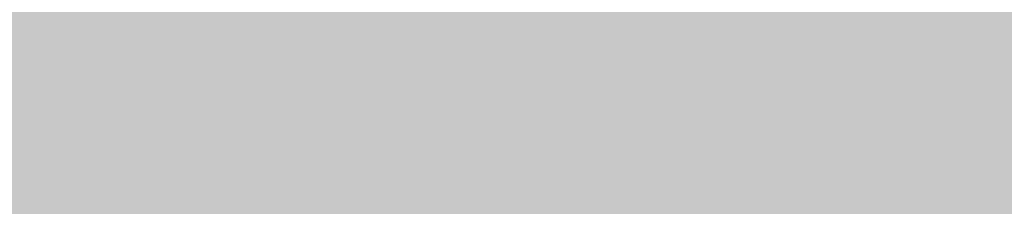
# Model space of a CAD drawing. Units: millimetres. Extents: x 0 to 2267, y 0 to 1823.
# Tile 49 of 256: x 1595.098 to 1596.855, y 1226.386 to 1226.718. Entities that reach past the tile are written whole.
import ezdxf

# ---------------------------------------------------------------- set-up
doc = ezdxf.new("R2010")
doc.units = ezdxf.units.MM
doc.header["$MEASUREMENT"] = 0
doc.layers.add('M-HATC', color=252, linetype='Continuous', lineweight=18)

msp = doc.modelspace()

# ---------------------------------------------------------------- hatches: boundary and pattern name
at = {"layer": 'M-HATC'}
h = msp.add_hatch(color=256, dxfattribs=at)
h.dxf.hatch_style = 1
h.paths.add_polyline_path([(2055.771, 1603.062), (1381.0868, 1603.062), (1381.0868, 1598.062), (2055.771, 1598.062)])
h.paths.add_polyline_path([(2055.771, 1598.062), (1381.0868, 1598.062), (1381.0868, 1593.062), (2055.771, 1593.062)])
h.paths.add_polyline_path([(2051.3074, 1536.7609), (1385.5504, 1536.7609), (1385.5504, 1526.7609), (1387.5504, 1526.7609), (1388.5366, 1525.0528), (1385.3319, 1521.2335), (1385.3319, 1521.2226), (2050.2542, 1522.7491), (2048.3212, 1525.0528), (2049.3074, 1526.7609), (2051.3074, 1526.7609)])
edge = h.paths.add_edge_path()
edge.add_arc((1847.5345, 1379.1492), 135, 222.603061, 222.890851, ccw=False)
edge.add_line((1748.1663, 1287.7656), (1683.0921, 1287.7656))
edge.add_arc((1583.7239, 1379.1492), 135, 317.109149, 317.396939, ccw=False)
edge.add_arc((1678.9686, 1290.6707), 5, 222.8909, 317.1091, ccw=False)
edge.add_arc((1774.2133, 1379.1492), 135, 222.603061, 222.890851, ccw=False)
edge.add_line((1674.8451, 1287.7656), (1609.7709, 1287.7656))
edge.add_arc((1510.4027, 1379.1492), 135, 317.109149, 317.396939, ccw=False)
edge.add_arc((1605.6474, 1290.6707), 5, 222.8909, 317.1091, ccw=False)
edge.add_arc((1700.8921, 1379.1492), 135, 222.603061, 222.890851, ccw=False)
edge.add_line((1601.5239, 1287.7656), (1536.4497, 1287.7656))
edge.add_arc((1437.0815, 1379.1492), 135, 317.109149, 317.396939, ccw=False)
edge.add_arc((1532.3262, 1290.6707), 5, 222.8909, 317.1091, ccw=False)
edge.add_arc((1627.5709, 1379.1492), 135, 222.603061, 222.890851, ccw=False)
edge.add_line((1528.2027, 1287.7656), (1505.9289, 1287.7656))
edge.add_spline(control_points=[(1505.9289, 1287.7656), (1504.2622, 1287.7656), (1504.2622, 1282.7656), (1505.9289, 1282.7656)], knot_values=[0, 0, 0, 0, 5, 5, 5, 5], degree=3, periodic=0)
edge.add_line((1505.9289, 1282.7656), (1930.9289, 1282.7656))
edge.add_spline(control_points=[(1930.9289, 1282.7656), (1932.5956, 1282.7656), (1932.5956, 1287.7656), (1930.9289, 1287.7656)], knot_values=[0, 0, 0, 0, 5, 5, 5, 5], degree=3, periodic=0)
edge.add_line((1930.9289, 1287.7656), (1903.0557, 1287.7656))
edge.add_arc((1803.6875, 1379.1492), 135, 317.109149, 317.396939, ccw=False)
edge.add_arc((1898.9322, 1290.6707), 5, 222.8909, 317.1091, ccw=False)
edge.add_arc((1994.1769, 1379.1492), 135, 222.603061, 222.890851, ccw=False)
edge.add_line((1894.8087, 1287.7656), (1829.7345, 1287.7656))
edge.add_arc((1730.3663, 1379.1492), 135, 317.109149, 317.396939, ccw=False)
edge.add_arc((1825.611, 1290.6707), 5, 222.8909, 317.1091, ccw=False)
edge.add_arc((1920.8557, 1379.1492), 135, 222.603061, 222.890851, ccw=False)
edge.add_line((1821.4875, 1287.7656), (1756.4133, 1287.7656))
edge.add_arc((1657.0451, 1379.1492), 135, 317.109149, 317.396939, ccw=False)
edge.add_arc((1752.2898, 1290.6707), 5, 222.8909, 317.1091, ccw=False)
edge = h.paths.add_edge_path()
edge.add_spline(control_points=[(1843.4289, 1227.2475), (1845.0956, 1227.2475), (1845.0956, 1232.2475), (1843.4289, 1232.2475)], knot_values=[0, 0, 0, 0, 5, 5, 5, 5], degree=3, periodic=0)
edge.add_line((1843.4289, 1232.2475), (1593.4289, 1232.2475))
edge.add_spline(control_points=[(1593.4289, 1232.2475), (1591.7622, 1232.2475), (1591.7622, 1227.2475), (1593.4289, 1227.2475)], knot_values=[0, 0, 0, 0, 5, 5, 5, 5], degree=3, periodic=0)
edge.add_line((1593.4289, 1227.2475), (1843.4289, 1227.2475))
h.paths.add_polyline_path([(1905.9289, 1127.4171), (1530.9289, 1127.4171, 0.414214), (1520.9289, 1117.4171), (1530.9289, 1117.4171), (1915.9289, 1117.4171, 0.414214)])
edge = h.paths.add_edge_path()
edge.add_arc((1397.0858, 1498.4078), 12.7299, 90.78215, 190.87871, ccw=False)
edge.add_line((1396.912, 1511.1365), (1428.0097, 1511.3488))
edge.add_line((1428.0097, 1511.3488), (1433.0097, 1511.3488))
edge.add_line((1433.0097, 1511.3488), (1434.439, 1511.3488))
edge.add_arc((1419.474, 1498.0804), 20, 41.561, 74.08211)
edge.add_line((1424.9592, 1517.3135), (1399.9351, 1517.2561))
edge.add_spline(control_points=[(1399.9307, 1517.2561), (1399.884, 1517.2131), (1399.8328, 1517.1689), (1399.7774, 1517.1236)], knot_values=[11.567499, 11.567499, 11.567499, 11.567499, 11.814249, 11.814249, 11.814249, 11.814249], degree=3, periodic=0)
edge.add_spline(control_points=[(1399.6328, 1517.0099), (1399.5831, 1516.9721), (1399.5307, 1516.9338), (1399.4759, 1516.8947)], knot_values=[11.167718, 11.167718, 11.167718, 11.167718, 11.365188, 11.365188, 11.365188, 11.365188], degree=3, periodic=0)
edge.add_spline(control_points=[(1399.3398, 1516.8001), (1399.1514, 1516.6719), (1398.9384, 1516.5377), (1398.704, 1516.3994)], knot_values=[10.376405, 10.376405, 10.376405, 10.376405, 11.00994, 11.00994, 11.00994, 11.00994], degree=3, periodic=0)
edge.add_spline(control_points=[(1398.6572, 1516.3719), (1398.5789, 1516.326), (1398.4983, 1516.2797), (1398.4155, 1516.2331)], knot_values=[10.125175, 10.125175, 10.125175, 10.125175, 10.334406, 10.334406, 10.334406, 10.334406], degree=3, periodic=0)
edge.add_spline(control_points=[(1398.2642, 1516.1487), (1398.196, 1516.1111), (1398.1263, 1516.0732), (1398.0555, 1516.0351)], knot_values=[9.832246, 9.832246, 9.832246, 9.832246, 9.999658, 9.999658, 9.999658, 9.999658], degree=3, periodic=0)
edge.add_spline(control_points=[(1397.9987, 1516.0048), (1397.7312, 1515.8621), (1397.446, 1515.7171), (1397.1466, 1515.5714)], knot_values=[9.161808, 9.161808, 9.161808, 9.161808, 9.787769, 9.787769, 9.787769, 9.787769], degree=3, periodic=0)
edge.add_spline(control_points=[(1397.1466, 1515.5714), (1396.8418, 1515.423), (1396.5222, 1515.274), (1396.1914, 1515.1262)], knot_values=[8.524455, 8.524455, 8.524455, 8.524455, 9.161808, 9.161808, 9.161808, 9.161808], degree=3, periodic=0)
edge.add_spline(control_points=[(1396.0777, 1515.0756), (1395.9854, 1515.0348), (1395.8922, 1514.994), (1395.7983, 1514.9534)], knot_values=[8.275193, 8.275193, 8.275193, 8.275193, 8.451726, 8.451726, 8.451726, 8.451726], degree=3, periodic=0)
edge.add_spline(control_points=[(1395.6018, 1514.8691), (1395.4997, 1514.8257), (1395.3968, 1514.7824), (1395.2932, 1514.7394)], knot_values=[7.962917, 7.962917, 7.962917, 7.962917, 8.152764, 8.152764, 8.152764, 8.152764], degree=3, periodic=0)
edge.add_spline(control_points=[(1395.2116, 1514.7057), (1394.8278, 1514.5475), (1394.4345, 1514.3929), (1394.0364, 1514.2442)], knot_values=[7.21254, 7.21254, 7.21254, 7.21254, 7.913148, 7.913148, 7.913148, 7.913148], degree=3, periodic=0)
edge.add_spline(control_points=[(1394.0364, 1514.2442), (1393.7076, 1514.1214), (1393.3754, 1514.0027), (1393.0427, 1513.8895)], knot_values=[6.633733, 6.633733, 6.633733, 6.633733, 7.21254, 7.21254, 7.21254, 7.21254], degree=3, periodic=0)
edge.add_spline(control_points=[(1392.8214, 1513.815), (1392.7198, 1513.7812), (1392.6181, 1513.7479), (1392.5166, 1513.7152)], knot_values=[6.328796, 6.328796, 6.328796, 6.328796, 6.505493, 6.505493, 6.505493, 6.505493], degree=3, periodic=0)
edge.add_spline(control_points=[(1392.5166, 1513.7152), (1392.3187, 1513.6515), (1392.1212, 1513.59), (1391.9244, 1513.531)], knot_values=[5.984605, 5.984605, 5.984605, 5.984605, 6.328796, 6.328796, 6.328796, 6.328796], degree=3, periodic=0)
edge.add_spline(control_points=[(1391.7915, 1513.4915), (1391.3122, 1513.3501), (1390.8384, 1513.2239), (1390.3784, 1513.1171)], knot_values=[5.066697, 5.066697, 5.066697, 5.066697, 5.907055, 5.907055, 5.907055, 5.907055], degree=3, periodic=0)
edge.add_spline(control_points=[(1390.3784, 1513.1171), (1390.1797, 1513.071), (1389.9836, 1513.0284), (1389.7907, 1512.9899)], knot_values=[4.70367, 4.70367, 4.70367, 4.70367, 5.066695, 5.066695, 5.066695, 5.066695], degree=3, periodic=0)
edge.add_spline(control_points=[(1389.422, 1512.9204), (1389.2459, 1512.8892), (1389.0729, 1512.8617), (1388.9036, 1512.8381)], knot_values=[4.130571, 4.130571, 4.130571, 4.130571, 4.469816, 4.469816, 4.469816, 4.469816], degree=3, periodic=0)
edge.add_spline(control_points=[(1388.9036, 1512.8381), (1388.591, 1512.7946), (1388.2911, 1512.7644), (1388.0071, 1512.7494)], knot_values=[3.504031, 3.504031, 3.504031, 3.504031, 4.130571, 4.130571, 4.130571, 4.130571], degree=3, periodic=0)
edge.add_spline(control_points=[(1387.9356, 1512.7459), (1387.8538, 1512.7423), (1387.7733, 1512.74), (1387.6944, 1512.739)], knot_values=[3.268866, 3.268866, 3.268866, 3.268866, 3.451164, 3.451164, 3.451164, 3.451164], degree=3, periodic=0)
edge.add_spline(control_points=[(1387.3351, 1512.7443), (1387.2076, 1512.7499), (1387.0847, 1512.7597), (1386.967, 1512.7739)], knot_values=[2.670686, 2.670686, 2.670686, 2.670686, 2.984, 2.984, 2.984, 2.984], degree=3, periodic=0)
edge.add_spline(control_points=[(1386.8327, 1512.7922), (1386.8209, 1512.7941), (1386.8092, 1512.7959), (1386.7975, 1512.7979)], knot_values=[2.516981, 2.516981, 2.516981, 2.516981, 2.549528, 2.549528, 2.549528, 2.549528], degree=3, periodic=0)
edge.add_spline(control_points=[(1386.4526, 1512.8735), (1386.4257, 1512.881), (1386.3993, 1512.889), (1386.3733, 1512.8972)], knot_values=[2.095869, 2.095869, 2.095869, 2.095869, 2.17941, 2.17941, 2.17941, 2.17941], degree=3, periodic=0)
edge.add_spline(control_points=[(1386.0691, 1513.0189), (1386.0634, 1513.0217), (1386.0577, 1513.0246), (1386.052, 1513.0275)], knot_values=[1.72453, 1.72453, 1.72453, 1.72453, 1.745933, 1.745933, 1.745933, 1.745933], degree=3, periodic=0)
edge.add_arc((1399.474, 1498.0804), 20, 131.82432, 180)
edge.add_arc((1630.3336, 1505.5484), 250.9708, 181.705176, 236.427975)
edge.add_arc((1605.3399, 1483.3044), 218.7822, 238.660829, 243.34961)
edge.add_arc((1647.0911, 1510.3592), 262.8986, 183.129836, 237.853442, ccw=False)
h.paths.add_polyline_path([(1406.5369, 1391.9644, 0.149382), (1491.5506, 1296.4418, -0.129517)], flags=17)
edge = h.paths.add_edge_path()
edge.add_arc((2037.3838, 1498.0804), 20, 0, 48.26587)
edge.add_spline(control_points=[(2050.6973, 1513.0052), (2050.6512, 1512.9847), (2050.6034, 1512.9655), (2050.5539, 1512.9477)], knot_values=[1.835652, 1.835652, 1.835652, 1.835652, 2.000781, 2.000781, 2.000781, 2.000781], degree=3, periodic=0)
edge.add_spline(control_points=[(2050.4616, 1512.9166), (2050.479, 1512.9221), (2050.4963, 1512.9277), (2050.5133, 1512.9335)], knot_values=[2.045477, 2.045477, 2.045477, 2.045477, 2.101389, 2.101389, 2.101389, 2.101389], degree=3, periodic=0)
edge.add_spline(control_points=[(2050.129, 1512.8342), (2050.1984, 1512.8473), (2050.2657, 1512.8623), (2050.3308, 1512.8792)], knot_values=[2.237629, 2.237629, 2.237629, 2.237629, 2.435841, 2.435841, 2.435841, 2.435841], degree=3, periodic=0)
edge.add_spline(control_points=[(2050.0946, 1512.8278), (2050.1061, 1512.8299), (2050.1176, 1512.832), (2050.129, 1512.8342)], knot_values=[2.435841, 2.435841, 2.435841, 2.435841, 2.468321, 2.468321, 2.468321, 2.468321], degree=3, periodic=0)
edge.add_spline(control_points=[(2049.7843, 1512.7851), (2049.8552, 1512.7922), (2049.9243, 1512.8008), (2049.9917, 1512.8109)], knot_values=[2.563852, 2.563852, 2.563852, 2.563852, 2.748541, 2.748541, 2.748541, 2.748541], degree=3, periodic=0)
edge.add_spline(control_points=[(2049.4052, 1512.7617), (2049.5364, 1512.7653), (2049.6629, 1512.773), (2049.7843, 1512.7851)], knot_values=[2.748541, 2.748541, 2.748541, 2.748541, 3.064882, 3.064882, 3.064882, 3.064882], degree=3, periodic=0)
edge.add_spline(control_points=[(2049.1698, 1512.7597), (2049.2336, 1512.7591), (2049.2965, 1512.7594), (2049.3584, 1512.7606)], knot_values=[3.102309, 3.102309, 3.102309, 3.102309, 3.2503, 3.2503, 3.2503, 3.2503], degree=3, periodic=0)
edge.add_spline(control_points=[(2048.8573, 1512.7691), (2048.9638, 1512.7638), (2049.068, 1512.7606), (2049.1698, 1512.7597)], knot_values=[3.2503, 3.2503, 3.2503, 3.2503, 3.486069, 3.486069, 3.486069, 3.486069], degree=3, periodic=0)
edge.add_spline(control_points=[(2048.6924, 1512.7789), (2048.3729, 1512.8009), (2048.0345, 1512.8411), (2047.6817, 1512.897)], knot_values=[3.606429, 3.606429, 3.606429, 3.606429, 4.2989, 4.2989, 4.2989, 4.2989], degree=3, periodic=0)
edge.add_spline(control_points=[(2047.6817, 1512.897), (2047.5458, 1512.9185), (2047.4077, 1512.9424), (2047.2678, 1512.9685)], knot_values=[4.2989, 4.2989, 4.2989, 4.2989, 4.565769, 4.565769, 4.565769, 4.565769], degree=3, periodic=0)
edge.add_spline(control_points=[(2047.2678, 1512.9685), (2047.1449, 1512.9914), (2047.0207, 1513.016), (2046.8951, 1513.0422)], knot_values=[4.565769, 4.565769, 4.565769, 4.565769, 4.799971, 4.799971, 4.799971, 4.799971], degree=3, periodic=0)
edge.add_spline(control_points=[(2046.8951, 1513.0422), (2046.5286, 1513.1188), (2046.1513, 1513.209), (2045.7676, 1513.3107)], knot_values=[4.799971, 4.799971, 4.799971, 4.799971, 5.483718, 5.483718, 5.483718, 5.483718], degree=3, periodic=0)
edge.add_spline(control_points=[(2045.7676, 1513.3107), (2045.3724, 1513.4154), (2044.9704, 1513.5322), (2044.5662, 1513.6588)], knot_values=[5.483718, 5.483718, 5.483718, 5.483718, 6.187866, 6.187866, 6.187866, 6.187866], degree=3, periodic=0)
edge.add_spline(control_points=[(2044.5662, 1513.6588), (2044.4149, 1513.7061), (2044.2633, 1513.7549), (2044.1116, 1513.8048)], knot_values=[6.187866, 6.187866, 6.187866, 6.187866, 6.451551, 6.451551, 6.451551, 6.451551], degree=3, periodic=0)
edge.add_spline(control_points=[(2044.1116, 1513.8048), (2043.9967, 1513.8427), (2043.8817, 1513.8813), (2043.7668, 1513.9205)], knot_values=[6.451551, 6.451551, 6.451551, 6.451551, 6.651434, 6.651434, 6.651434, 6.651434], degree=3, periodic=0)
edge.add_spline(control_points=[(2043.7668, 1513.9205), (2043.3716, 1514.0554), (2042.9774, 1514.1979), (2042.5886, 1514.3458)], knot_values=[6.651434, 6.651434, 6.651434, 6.651434, 7.338879, 7.338879, 7.338879, 7.338879], degree=3, periodic=0)
edge.add_spline(control_points=[(2042.5886, 1514.3458), (2042.1643, 1514.5071), (2041.7465, 1514.6749), (2041.3409, 1514.846)], knot_values=[7.338879, 7.338879, 7.338879, 7.338879, 8.089209, 8.089209, 8.089209, 8.089209], degree=3, periodic=0)
edge.add_spline(control_points=[(2041.3409, 1514.846), (2041.1028, 1514.9465), (2040.869, 1515.0481), (2040.6405, 1515.1502)], knot_values=[8.089209, 8.089209, 8.089209, 8.089209, 8.529587, 8.529587, 8.529587, 8.529587], degree=3, periodic=0)
edge.add_spline(control_points=[(2040.51, 1515.2089), (2040.0824, 1515.4022), (2039.6747, 1515.5971), (2039.295, 1515.7894)], knot_values=[8.613818, 8.613818, 8.613818, 8.613818, 9.44571, 9.44571, 9.44571, 9.44571], degree=3, periodic=0)
edge.add_spline(control_points=[(2039.295, 1515.7894), (2039.0618, 1515.9075), (2038.8391, 1516.0246), (2038.6288, 1516.1398)], knot_values=[9.44571, 9.44571, 9.44571, 9.44571, 9.956404, 9.956404, 9.956404, 9.956404], degree=3, periodic=0)
edge.add_spline(control_points=[(2038.6288, 1516.1398), (2038.5187, 1516.2001), (2038.4121, 1516.2598), (2038.309, 1516.3189)], knot_values=[9.956404, 9.956404, 9.956404, 9.956404, 10.223542, 10.223542, 10.223542, 10.223542], degree=3, periodic=0)
edge.add_spline(control_points=[(2038.309, 1516.3189), (2038.2138, 1516.3735), (2038.1216, 1516.4276), (2038.0328, 1516.481)], knot_values=[10.223542, 10.223542, 10.223542, 10.223542, 10.47051, 10.47051, 10.47051, 10.47051], degree=3, periodic=0)
edge.add_spline(control_points=[(2038.0328, 1516.481), (2037.7855, 1516.6296), (2037.5639, 1516.773), (2037.3722, 1516.909)], knot_values=[10.47051, 10.47051, 10.47051, 10.47051, 11.15767, 11.15767, 11.15767, 11.15767], degree=3, periodic=0)
edge.add_spline(control_points=[(2037.3722, 1516.909), (2037.2789, 1516.9752), (2037.1927, 1517.0396), (2037.1142, 1517.102)], knot_values=[11.15767, 11.15767, 11.15767, 11.15767, 11.49227, 11.49227, 11.49227, 11.49227], degree=3, periodic=0)
edge.add_spline(control_points=[(2036.8564, 1517.3259), (2036.9148, 1517.2692), (2036.9814, 1517.2103), (2037.0557, 1517.1492)], knot_values=[11.577341, 11.577341, 11.577341, 11.577341, 11.91035, 11.91035, 11.91035, 11.91035], degree=3, periodic=0)
edge.add_spline(control_points=[(2036.8074, 1517.3748), (2036.823, 1517.3587), (2036.8393, 1517.3424), (2036.8564, 1517.3259)], knot_values=[11.91035, 11.91035, 11.91035, 11.91035, 12.007402, 12.007402, 12.007402, 12.007402], degree=3, periodic=0)
edge.add_spline(control_points=[(2036.7017, 1517.494), (2036.7104, 1517.483), (2036.7196, 1517.4719), (2036.7291, 1517.4606)], knot_values=[12.184155, 12.184155, 12.184155, 12.184155, 12.255409, 12.255409, 12.255409, 12.255409], degree=3, periodic=0)
edge.add_spline(control_points=[(2036.6159, 1517.6205), (2036.62, 1517.613), (2036.6243, 1517.6055), (2036.6289, 1517.5979)], knot_values=[12.487913, 12.487913, 12.487913, 12.487913, 12.541035, 12.541035, 12.541035, 12.541035], degree=3, periodic=0)
edge.add_spline(control_points=[(2036.5635, 1517.786), (2036.5637, 1517.7794), (2036.5642, 1517.7726), (2036.565, 1517.7658)], knot_values=[12.911761, 12.911761, 12.911761, 12.911761, 12.968286, 12.968286, 12.968286, 12.968286], degree=3, periodic=0)
edge.add_spline(control_points=[(2036.6166, 1517.9304), (2036.6125, 1517.9259), (2036.6086, 1517.9212), (2036.6049, 1517.9165)], knot_values=[13.382527, 13.382527, 13.382527, 13.382527, 13.433791, 13.433791, 13.433791, 13.433791], degree=3, periodic=0)
edge.add_spline(control_points=[(2036.749, 1518.017), (2036.7361, 1518.0116), (2036.7239, 1518.006), (2036.7124, 1518.0002)], knot_values=[13.726299, 13.726299, 13.726299, 13.726299, 13.809928, 13.809928, 13.809928, 13.809928], degree=3, periodic=0)
edge.add_spline(control_points=[(2036.8604, 1518.0528), (2036.8386, 1518.0474), (2036.8181, 1518.0416), (2036.7988, 1518.0353)], knot_values=[13.910887, 13.910887, 13.910887, 13.910887, 14.02153, 14.02153, 14.02153, 14.02153], degree=3, periodic=0)
edge.add_line((2036.9639, 1518.0804), (2032.3838, 1518.0804))
edge.add_line((2032.3838, 1518.0804), (2027.3838, 1518.0804))
edge.add_line((2027.3838, 1518.0804), (2022.3838, 1518.0804))
edge.add_line((2022.3838, 1518.0804), (2017.3838, 1518.0804))
edge.add_arc((2017.3838, 1498.0804), 20, 90, 138.439)
edge.add_line((2002.4188, 1511.3488), (2003.8481, 1511.3488))
edge.add_line((2003.8481, 1511.3488), (2008.8481, 1511.3488))
edge.add_line((2008.8481, 1511.3488), (2039.772, 1511.1377))
edge.add_arc((2039.772, 1498.4078), 12.7299, -10.87871, 90, ccw=False)
edge.add_arc((1789.7668, 1510.3592), 262.8986, 302.146558, 356.870164, ccw=False)
edge.add_arc((1831.5179, 1483.3044), 218.7822, 296.65039, 301.339171)
edge.add_arc((1806.5242, 1505.5484), 250.9708, 303.572025, 358.294824)
h.paths.add_polyline_path([(2030.321, 1391.9644, -0.129517), (1945.3072, 1296.4418, 0.149382)], flags=17)
edge = h.paths.add_edge_path()
edge.add_spline(control_points=[(2037.2464, 1518.0821), (2037.2898, 1518.081), (2037.3355, 1518.0804), (2037.3838, 1518.0804)], knot_values=[0.000012, 0.000012, 0.000012, 0.000012, 0.144754, 0.144754, 0.144754, 0.144754], degree=3, periodic=0)
edge.add_line((2037.3357, 1518.0804), (2037.0096, 1518.0804))
edge.add_spline(control_points=[(2037.0096, 1518.0804), (2036.9822, 1518.0768), (2036.956, 1518.0727), (2036.9312, 1518.0681)], knot_values=[14.13465, 14.13465, 14.13465, 14.13465, 14.247197, 14.247197, 14.247197, 14.247197], degree=3, periodic=0)
edge.add_spline(control_points=[(2036.9312, 1518.0681), (2036.9276, 1518.0674), (2036.9241, 1518.0667), (2036.9205, 1518.0661)], knot_values=[14.118315, 14.118315, 14.118315, 14.118315, 14.13465, 14.13465, 14.13465, 14.13465], degree=3, periodic=0)
edge.add_spline(control_points=[(2036.9205, 1518.0661), (2036.9118, 1518.0644), (2036.9032, 1518.0626), (2036.8948, 1518.0608)], knot_values=[14.078086, 14.078086, 14.078086, 14.078086, 14.118315, 14.118315, 14.118315, 14.118315], degree=3, periodic=0)
edge.add_spline(control_points=[(2036.8948, 1518.0608), (2036.883, 1518.0583), (2036.8716, 1518.0556), (2036.8604, 1518.0528)], knot_values=[14.02153, 14.02153, 14.02153, 14.02153, 14.078086, 14.078086, 14.078086, 14.078086], degree=3, periodic=0)
edge.add_spline(control_points=[(2036.8604, 1518.0528), (2036.8386, 1518.0474), (2036.8181, 1518.0416), (2036.7988, 1518.0353)], knot_values=[13.910887, 13.910887, 13.910887, 13.910887, 14.02153, 14.02153, 14.02153, 14.02153], degree=3, periodic=0)
edge.add_spline(control_points=[(2036.7988, 1518.0353), (2036.7981, 1518.035), (2036.7974, 1518.0348), (2036.7967, 1518.0346)], knot_values=[13.906906, 13.906906, 13.906906, 13.906906, 13.910887, 13.910887, 13.910887, 13.910887], degree=3, periodic=0)
edge.add_spline(control_points=[(2036.7967, 1518.0346), (2036.7882, 1518.0318), (2036.7799, 1518.0289), (2036.7719, 1518.0259)], knot_values=[13.857826, 13.857826, 13.857826, 13.857826, 13.906906, 13.906906, 13.906906, 13.906906], degree=3, periodic=0)
edge.add_spline(control_points=[(2036.7719, 1518.0259), (2036.764, 1518.023), (2036.7564, 1518.02), (2036.749, 1518.017)], knot_values=[13.809928, 13.809928, 13.809928, 13.809928, 13.857826, 13.857826, 13.857826, 13.857826], degree=3, periodic=0)
edge.add_spline(control_points=[(2036.749, 1518.017), (2036.7361, 1518.0116), (2036.7239, 1518.006), (2036.7124, 1518.0002)], knot_values=[13.726299, 13.726299, 13.726299, 13.726299, 13.809928, 13.809928, 13.809928, 13.809928], degree=3, periodic=0)
edge.add_spline(control_points=[(2036.7124, 1518.0002), (2036.7121, 1518), (2036.7118, 1517.9999), (2036.7115, 1517.9997)], knot_values=[13.723993, 13.723993, 13.723993, 13.723993, 13.726299, 13.726299, 13.726299, 13.726299], degree=3, periodic=0)
edge.add_spline(control_points=[(2036.7115, 1517.9997), (2036.7063, 1517.9971), (2036.7013, 1517.9944), (2036.6965, 1517.9917)], knot_values=[13.686536, 13.686536, 13.686536, 13.686536, 13.723993, 13.723993, 13.723993, 13.723993], degree=3, periodic=0)
edge.add_spline(control_points=[(2036.6965, 1517.9917), (2036.6919, 1517.9891), (2036.6874, 1517.9865), (2036.6831, 1517.9839)], knot_values=[13.651251, 13.651251, 13.651251, 13.651251, 13.686536, 13.686536, 13.686536, 13.686536], degree=3, periodic=0)
edge.add_spline(control_points=[(2036.6831, 1517.9839), (2036.6764, 1517.9798), (2036.67, 1517.9757), (2036.6639, 1517.9714)], knot_values=[13.596804, 13.596804, 13.596804, 13.596804, 13.651251, 13.651251, 13.651251, 13.651251], degree=3, periodic=0)
edge.add_spline(control_points=[(2036.6639, 1517.9714), (2036.6636, 1517.9712), (2036.6633, 1517.9709), (2036.6629, 1517.9707)], knot_values=[13.593956, 13.593956, 13.593956, 13.593956, 13.596804, 13.596804, 13.596804, 13.596804], degree=3, periodic=0)
edge.add_spline(control_points=[(2036.6629, 1517.9707), (2036.6603, 1517.9689), (2036.6577, 1517.967), (2036.6552, 1517.9651)], knot_values=[13.570322, 13.570322, 13.570322, 13.570322, 13.593956, 13.593956, 13.593956, 13.593956], degree=3, periodic=0)
edge.add_spline(control_points=[(2036.6552, 1517.9651), (2036.6525, 1517.9631), (2036.6499, 1517.9611), (2036.6474, 1517.9591)], knot_values=[13.545477, 13.545477, 13.545477, 13.545477, 13.570322, 13.570322, 13.570322, 13.570322], degree=3, periodic=0)
edge.add_spline(control_points=[(2036.6474, 1517.9591), (2036.6472, 1517.9589), (2036.6471, 1517.9588), (2036.6469, 1517.9587)], knot_values=[13.543931, 13.543931, 13.543931, 13.543931, 13.545477, 13.545477, 13.545477, 13.545477], degree=3, periodic=0)
edge.add_spline(control_points=[(2036.6469, 1517.9587), (2036.6412, 1517.9541), (2036.6358, 1517.9494), (2036.6307, 1517.9447)], knot_values=[13.488237, 13.488237, 13.488237, 13.488237, 13.543931, 13.543931, 13.543931, 13.543931], degree=3, periodic=0)
edge.add_spline(control_points=[(2036.6307, 1517.9447), (2036.6282, 1517.9423), (2036.6257, 1517.9399), (2036.6233, 1517.9374)], knot_values=[13.460307, 13.460307, 13.460307, 13.460307, 13.488237, 13.488237, 13.488237, 13.488237], degree=3, periodic=0)
edge.add_spline(control_points=[(2036.6233, 1517.9374), (2036.6215, 1517.9356), (2036.6198, 1517.9338), (2036.6181, 1517.932)], knot_values=[13.439712, 13.439712, 13.439712, 13.439712, 13.460307, 13.460307, 13.460307, 13.460307], degree=3, periodic=0)
edge.add_spline(control_points=[(2036.6181, 1517.932), (2036.6176, 1517.9315), (2036.6171, 1517.9309), (2036.6166, 1517.9304)], knot_values=[13.433791, 13.433791, 13.433791, 13.433791, 13.439712, 13.439712, 13.439712, 13.439712], degree=3, periodic=0)
edge.add_spline(control_points=[(2036.6166, 1517.9304), (2036.6125, 1517.9259), (2036.6086, 1517.9212), (2036.6049, 1517.9165)], knot_values=[13.382527, 13.382527, 13.382527, 13.382527, 13.433791, 13.433791, 13.433791, 13.433791], degree=3, periodic=0)
edge.add_spline(control_points=[(2036.6049, 1517.9165), (2036.6026, 1517.9135), (2036.6004, 1517.9104), (2036.5982, 1517.9074)], knot_values=[13.350017, 13.350017, 13.350017, 13.350017, 13.382527, 13.382527, 13.382527, 13.382527], degree=3, periodic=0)
edge.add_spline(control_points=[(2036.5982, 1517.9074), (2036.5972, 1517.9059), (2036.5962, 1517.9043), (2036.5952, 1517.9028)], knot_values=[13.333922, 13.333922, 13.333922, 13.333922, 13.350017, 13.350017, 13.350017, 13.350017], degree=3, periodic=0)
edge.add_spline(control_points=[(2036.5952, 1517.9028), (2036.5945, 1517.9018), (2036.5939, 1517.9009), (2036.5933, 1517.8999)], knot_values=[13.323828, 13.323828, 13.323828, 13.323828, 13.333922, 13.333922, 13.333922, 13.333922], degree=3, periodic=0)
edge.add_spline(control_points=[(2036.5933, 1517.8999), (2036.5905, 1517.8955), (2036.5879, 1517.8909), (2036.5855, 1517.8864)], knot_values=[13.277545, 13.277545, 13.277545, 13.277545, 13.323828, 13.323828, 13.323828, 13.323828], degree=3, periodic=0)
edge.add_spline(control_points=[(2036.5855, 1517.8864), (2036.5836, 1517.8827), (2036.5817, 1517.8789), (2036.5801, 1517.8751)], knot_values=[13.240119, 13.240119, 13.240119, 13.240119, 13.277545, 13.277545, 13.277545, 13.277545], degree=3, periodic=0)
edge.add_spline(control_points=[(2036.5801, 1517.8751), (2036.5795, 1517.8739), (2036.579, 1517.8727), (2036.5785, 1517.8715)], knot_values=[13.228211, 13.228211, 13.228211, 13.228211, 13.240119, 13.240119, 13.240119, 13.240119], degree=3, periodic=0)
edge.add_spline(control_points=[(2036.5785, 1517.8715), (2036.578, 1517.8702), (2036.5774, 1517.869), (2036.5769, 1517.8677)], knot_values=[13.215717, 13.215717, 13.215717, 13.215717, 13.228211, 13.228211, 13.228211, 13.228211], degree=3, periodic=0)
edge.add_spline(control_points=[(2036.5769, 1517.8677), (2036.5755, 1517.864), (2036.5741, 1517.8603), (2036.5729, 1517.8565)], knot_values=[13.179847, 13.179847, 13.179847, 13.179847, 13.215717, 13.215717, 13.215717, 13.215717], degree=3, periodic=0)
edge.add_spline(control_points=[(2036.5729, 1517.8565), (2036.5713, 1517.8515), (2036.5699, 1517.8464), (2036.5687, 1517.8413)], knot_values=[13.132017, 13.132017, 13.132017, 13.132017, 13.179847, 13.179847, 13.179847, 13.179847], degree=3, periodic=0)
edge.add_spline(control_points=[(2036.5687, 1517.8413), (2036.5684, 1517.8402), (2036.5682, 1517.8392), (2036.568, 1517.8382)], knot_values=[13.122482, 13.122482, 13.122482, 13.122482, 13.132017, 13.132017, 13.132017, 13.132017], degree=3, periodic=0)
edge.add_spline(control_points=[(2036.568, 1517.8382), (2036.5676, 1517.8363), (2036.5672, 1517.8345), (2036.5669, 1517.8327)], knot_values=[13.105592, 13.105592, 13.105592, 13.105592, 13.122482, 13.122482, 13.122482, 13.122482], degree=3, periodic=0)
edge.add_spline(control_points=[(2036.5669, 1517.8327), (2036.5662, 1517.8292), (2036.5657, 1517.8257), (2036.5652, 1517.8222)], knot_values=[13.074063, 13.074063, 13.074063, 13.074063, 13.105592, 13.105592, 13.105592, 13.105592], degree=3, periodic=0)
edge.add_spline(control_points=[(2036.5652, 1517.8222), (2036.5652, 1517.8222), (2036.5652, 1517.8222), (2036.5652, 1517.8222)], knot_values=[13.074043, 13.074043, 13.074043, 13.074043, 13.074063, 13.074063, 13.074063, 13.074063], degree=3, periodic=0)
edge.add_spline(control_points=[(2036.5652, 1517.8222), (2036.5644, 1517.8164), (2036.5639, 1517.8106), (2036.5636, 1517.8046)], knot_values=[13.021884, 13.021884, 13.021884, 13.021884, 13.074043, 13.074043, 13.074043, 13.074043], degree=3, periodic=0)
edge.add_spline(control_points=[(2036.5636, 1517.8046), (2036.5636, 1517.804), (2036.5636, 1517.8034), (2036.5635, 1517.8028)], knot_values=[13.01674, 13.01674, 13.01674, 13.01674, 13.021884, 13.021884, 13.021884, 13.021884], degree=3, periodic=0)
edge.add_spline(control_points=[(2036.5635, 1517.8028), (2036.5634, 1517.8005), (2036.5634, 1517.7982), (2036.5634, 1517.7958)], knot_values=[12.996438, 12.996438, 12.996438, 12.996438, 13.01674, 13.01674, 13.01674, 13.01674], degree=3, periodic=0)
edge.add_spline(control_points=[(2036.5634, 1517.7958), (2036.5633, 1517.7926), (2036.5634, 1517.7893), (2036.5635, 1517.786)], knot_values=[12.968286, 12.968286, 12.968286, 12.968286, 12.996438, 12.996438, 12.996438, 12.996438], degree=3, periodic=0)
edge.add_spline(control_points=[(2036.5635, 1517.786), (2036.5637, 1517.7794), (2036.5642, 1517.7726), (2036.565, 1517.7658)], knot_values=[12.911761, 12.911761, 12.911761, 12.911761, 12.968286, 12.968286, 12.968286, 12.968286], degree=3, periodic=0)
edge.add_spline(control_points=[(2036.565, 1517.7658), (2036.565, 1517.7657), (2036.565, 1517.7656), (2036.565, 1517.7656)], knot_values=[12.911017, 12.911017, 12.911017, 12.911017, 12.911761, 12.911761, 12.911761, 12.911761], degree=3, periodic=0)
edge.add_spline(control_points=[(2036.565, 1517.7656), (2036.5654, 1517.7625), (2036.5658, 1517.7593), (2036.5663, 1517.7562)], knot_values=[12.88528, 12.88528, 12.88528, 12.88528, 12.911017, 12.911017, 12.911017, 12.911017], degree=3, periodic=0)
edge.add_spline(control_points=[(2036.5663, 1517.7562), (2036.5667, 1517.7534), (2036.5672, 1517.7506), (2036.5677, 1517.7478)], knot_values=[12.862519, 12.862519, 12.862519, 12.862519, 12.88528, 12.88528, 12.88528, 12.88528], degree=3, periodic=0)
edge.add_spline(control_points=[(2036.5677, 1517.7478), (2036.5678, 1517.7474), (2036.5679, 1517.7469), (2036.568, 1517.7465)], knot_values=[12.858885, 12.858885, 12.858885, 12.858885, 12.862519, 12.862519, 12.862519, 12.862519], degree=3, periodic=0)
edge.add_spline(control_points=[(2036.568, 1517.7465), (2036.5692, 1517.7399), (2036.5707, 1517.7332), (2036.5724, 1517.7264)], knot_values=[12.8053, 12.8053, 12.8053, 12.8053, 12.858885, 12.858885, 12.858885, 12.858885], degree=3, periodic=0)
edge.add_spline(control_points=[(2036.5724, 1517.7264), (2036.5734, 1517.7226), (2036.5745, 1517.7187), (2036.5756, 1517.7149)], knot_values=[12.775176, 12.775176, 12.775176, 12.775176, 12.8053, 12.8053, 12.8053, 12.8053], degree=3, periodic=0)
edge.add_spline(control_points=[(2036.5756, 1517.7149), (2036.5763, 1517.7125), (2036.577, 1517.7102), (2036.5778, 1517.7078)], knot_values=[12.756759, 12.756759, 12.756759, 12.756759, 12.775176, 12.775176, 12.775176, 12.775176], degree=3, periodic=0)
edge.add_spline(control_points=[(2036.5778, 1517.7078), (2036.5781, 1517.7067), (2036.5784, 1517.7057), (2036.5787, 1517.7047)], knot_values=[12.748742, 12.748742, 12.748742, 12.748742, 12.756759, 12.756759, 12.756759, 12.756759], degree=3, periodic=0)
edge.add_spline(control_points=[(2036.5787, 1517.7047), (2036.5808, 1517.6983), (2036.5831, 1517.6919), (2036.5856, 1517.6854)], knot_values=[12.69959, 12.69959, 12.69959, 12.69959, 12.748742, 12.748742, 12.748742, 12.748742], degree=3, periodic=0)
edge.add_spline(control_points=[(2036.5856, 1517.6854), (2036.5876, 1517.68), (2036.5898, 1517.6746), (2036.5921, 1517.6692)], knot_values=[12.659038, 12.659038, 12.659038, 12.659038, 12.69959, 12.69959, 12.69959, 12.69959], degree=3, periodic=0)
edge.add_spline(control_points=[(2036.5921, 1517.6692), (2036.594, 1517.6648), (2036.5959, 1517.6605), (2036.5979, 1517.6561)], knot_values=[12.626806, 12.626806, 12.626806, 12.626806, 12.659038, 12.659038, 12.659038, 12.659038], degree=3, periodic=0)
edge.add_spline(control_points=[(2036.5979, 1517.6561), (2036.5984, 1517.6551), (2036.5989, 1517.6541), (2036.5993, 1517.6531)], knot_values=[12.619394, 12.619394, 12.619394, 12.619394, 12.626806, 12.626806, 12.626806, 12.626806], degree=3, periodic=0)
edge.add_spline(control_points=[(2036.5993, 1517.6531), (2036.6043, 1517.6424), (2036.6099, 1517.6315), (2036.6159, 1517.6205)], knot_values=[12.541039, 12.541039, 12.541039, 12.541039, 12.619394, 12.619394, 12.619394, 12.619394], degree=3, periodic=0)
edge.add_spline(control_points=[(2036.6159, 1517.6205), (2036.6159, 1517.6205), (2036.6159, 1517.6205), (2036.6159, 1517.6205)], knot_values=[12.541035, 12.541035, 12.541035, 12.541035, 12.541039, 12.541039, 12.541039, 12.541039], degree=3, periodic=0)
edge.add_spline(control_points=[(2036.6159, 1517.6205), (2036.62, 1517.613), (2036.6243, 1517.6055), (2036.6289, 1517.5979)], knot_values=[12.487913, 12.487913, 12.487913, 12.487913, 12.541035, 12.541035, 12.541035, 12.541035], degree=3, periodic=0)
edge.add_spline(control_points=[(2036.6289, 1517.5979), (2036.6326, 1517.5916), (2036.6365, 1517.5853), (2036.6406, 1517.5789)], knot_values=[12.443982, 12.443982, 12.443982, 12.443982, 12.487913, 12.487913, 12.487913, 12.487913], degree=3, periodic=0)
edge.add_spline(control_points=[(2036.6406, 1517.5789), (2036.6414, 1517.5776), (2036.6423, 1517.5763), (2036.6431, 1517.5749)], knot_values=[12.434996, 12.434996, 12.434996, 12.434996, 12.443982, 12.443982, 12.443982, 12.443982], degree=3, periodic=0)
edge.add_spline(control_points=[(2036.6431, 1517.5749), (2036.6531, 1517.5596), (2036.6639, 1517.5439), (2036.6756, 1517.528)], knot_values=[12.329647, 12.329647, 12.329647, 12.329647, 12.434996, 12.434996, 12.434996, 12.434996], degree=3, periodic=0)
edge.add_spline(control_points=[(2036.6756, 1517.528), (2036.6839, 1517.5168), (2036.6925, 1517.5055), (2036.7017, 1517.494)], knot_values=[12.255409, 12.255409, 12.255409, 12.255409, 12.329647, 12.329647, 12.329647, 12.329647], degree=3, periodic=0)
edge.add_spline(control_points=[(2036.7017, 1517.494), (2036.7104, 1517.483), (2036.7196, 1517.4719), (2036.7291, 1517.4606)], knot_values=[12.184155, 12.184155, 12.184155, 12.184155, 12.255409, 12.255409, 12.255409, 12.255409], degree=3, periodic=0)
edge.add_spline(control_points=[(2036.7291, 1517.4606), (2036.7436, 1517.4435), (2036.759, 1517.4262), (2036.7753, 1517.4085)], knot_values=[12.075961, 12.075961, 12.075961, 12.075961, 12.184155, 12.184155, 12.184155, 12.184155], degree=3, periodic=0)
edge.add_spline(control_points=[(2036.7753, 1517.4085), (2036.7763, 1517.4075), (2036.7773, 1517.4064), (2036.7783, 1517.4054)], knot_values=[12.069502, 12.069502, 12.069502, 12.069502, 12.075961, 12.075961, 12.075961, 12.075961], degree=3, periodic=0)
edge.add_spline(control_points=[(2036.7783, 1517.4054), (2036.7877, 1517.3953), (2036.7974, 1517.385), (2036.8074, 1517.3748)], knot_values=[12.007402, 12.007402, 12.007402, 12.007402, 12.069502, 12.069502, 12.069502, 12.069502], degree=3, periodic=0)
edge.add_spline(control_points=[(2036.8074, 1517.3748), (2036.823, 1517.3587), (2036.8393, 1517.3424), (2036.8564, 1517.3259)], knot_values=[11.91035, 11.91035, 11.91035, 11.91035, 12.007402, 12.007402, 12.007402, 12.007402], degree=3, periodic=0)
edge.add_spline(control_points=[(2036.8564, 1517.3259), (2036.9148, 1517.2692), (2036.9814, 1517.2103), (2037.0557, 1517.1492)], knot_values=[11.577341, 11.577341, 11.577341, 11.577341, 11.91035, 11.91035, 11.91035, 11.91035], degree=3, periodic=0)
edge.add_spline(control_points=[(2037.0557, 1517.1492), (2037.0747, 1517.1336), (2037.0942, 1517.1179), (2037.1142, 1517.102)], knot_values=[11.49227, 11.49227, 11.49227, 11.49227, 11.577341, 11.577341, 11.577341, 11.577341], degree=3, periodic=0)
edge.add_spline(control_points=[(2037.1142, 1517.102), (2037.1927, 1517.0396), (2037.2789, 1516.9752), (2037.3722, 1516.909)], knot_values=[11.15767, 11.15767, 11.15767, 11.15767, 11.49227, 11.49227, 11.49227, 11.49227], degree=3, periodic=0)
edge.add_spline(control_points=[(2037.3722, 1516.909), (2037.5639, 1516.773), (2037.7855, 1516.6296), (2038.0328, 1516.481)], knot_values=[10.47051, 10.47051, 10.47051, 10.47051, 11.15767, 11.15767, 11.15767, 11.15767], degree=3, periodic=0)
edge.add_spline(control_points=[(2038.0328, 1516.481), (2038.1216, 1516.4276), (2038.2138, 1516.3735), (2038.309, 1516.3189)], knot_values=[10.223542, 10.223542, 10.223542, 10.223542, 10.47051, 10.47051, 10.47051, 10.47051], degree=3, periodic=0)
edge.add_spline(control_points=[(2038.309, 1516.3189), (2038.4121, 1516.2598), (2038.5187, 1516.2001), (2038.6288, 1516.1398)], knot_values=[9.956404, 9.956404, 9.956404, 9.956404, 10.223542, 10.223542, 10.223542, 10.223542], degree=3, periodic=0)
edge.add_spline(control_points=[(2038.6288, 1516.1398), (2038.8391, 1516.0246), (2039.0618, 1515.9075), (2039.295, 1515.7894)], knot_values=[9.44571, 9.44571, 9.44571, 9.44571, 9.956404, 9.956404, 9.956404, 9.956404], degree=3, periodic=0)
edge.add_spline(control_points=[(2039.295, 1515.7894), (2039.6747, 1515.5971), (2040.0824, 1515.4022), (2040.51, 1515.2089)], knot_values=[8.613818, 8.613818, 8.613818, 8.613818, 9.44571, 9.44571, 9.44571, 9.44571], degree=3, periodic=0)
edge.add_spline(control_points=[(2040.51, 1515.2089), (2040.5533, 1515.1893), (2040.5968, 1515.1697), (2040.6405, 1515.1502)], knot_values=[8.529587, 8.529587, 8.529587, 8.529587, 8.613818, 8.613818, 8.613818, 8.613818], degree=3, periodic=0)
edge.add_spline(control_points=[(2040.6405, 1515.1502), (2040.869, 1515.0481), (2041.1028, 1514.9465), (2041.3409, 1514.846)], knot_values=[8.089209, 8.089209, 8.089209, 8.089209, 8.529587, 8.529587, 8.529587, 8.529587], degree=3, periodic=0)
edge.add_spline(control_points=[(2041.3409, 1514.846), (2041.7465, 1514.6749), (2042.1643, 1514.5071), (2042.5886, 1514.3458)], knot_values=[7.338879, 7.338879, 7.338879, 7.338879, 8.089209, 8.089209, 8.089209, 8.089209], degree=3, periodic=0)
edge.add_spline(control_points=[(2042.5886, 1514.3458), (2042.9774, 1514.1979), (2043.3716, 1514.0554), (2043.7668, 1513.9205)], knot_values=[6.651434, 6.651434, 6.651434, 6.651434, 7.338879, 7.338879, 7.338879, 7.338879], degree=3, periodic=0)
edge.add_spline(control_points=[(2043.7668, 1513.9205), (2043.8817, 1513.8813), (2043.9967, 1513.8427), (2044.1116, 1513.8048)], knot_values=[6.451551, 6.451551, 6.451551, 6.451551, 6.651434, 6.651434, 6.651434, 6.651434], degree=3, periodic=0)
edge.add_spline(control_points=[(2044.1116, 1513.8048), (2044.2633, 1513.7549), (2044.4149, 1513.7061), (2044.5662, 1513.6588)], knot_values=[6.187866, 6.187866, 6.187866, 6.187866, 6.451551, 6.451551, 6.451551, 6.451551], degree=3, periodic=0)
edge.add_spline(control_points=[(2044.5662, 1513.6588), (2044.9704, 1513.5322), (2045.3724, 1513.4154), (2045.7676, 1513.3107)], knot_values=[5.483718, 5.483718, 5.483718, 5.483718, 6.187866, 6.187866, 6.187866, 6.187866], degree=3, periodic=0)
edge.add_spline(control_points=[(2045.7676, 1513.3107), (2046.1513, 1513.209), (2046.5286, 1513.1188), (2046.8951, 1513.0422)], knot_values=[4.799971, 4.799971, 4.799971, 4.799971, 5.483718, 5.483718, 5.483718, 5.483718], degree=3, periodic=0)
edge.add_spline(control_points=[(2046.8951, 1513.0422), (2047.0207, 1513.016), (2047.1449, 1512.9914), (2047.2678, 1512.9685)], knot_values=[4.565769, 4.565769, 4.565769, 4.565769, 4.799971, 4.799971, 4.799971, 4.799971], degree=3, periodic=0)
edge.add_spline(control_points=[(2047.2678, 1512.9685), (2047.4077, 1512.9424), (2047.5458, 1512.9185), (2047.6817, 1512.897)], knot_values=[4.2989, 4.2989, 4.2989, 4.2989, 4.565769, 4.565769, 4.565769, 4.565769], degree=3, periodic=0)
edge.add_spline(control_points=[(2047.6817, 1512.897), (2048.0345, 1512.8411), (2048.3729, 1512.8009), (2048.6924, 1512.7789)], knot_values=[3.606429, 3.606429, 3.606429, 3.606429, 4.2989, 4.2989, 4.2989, 4.2989], degree=3, periodic=0)
edge.add_spline(control_points=[(2048.6924, 1512.7789), (2048.7479, 1512.7751), (2048.8029, 1512.7718), (2048.8573, 1512.7691)], knot_values=[3.486069, 3.486069, 3.486069, 3.486069, 3.606429, 3.606429, 3.606429, 3.606429], degree=3, periodic=0)
edge.add_spline(control_points=[(2048.8573, 1512.7691), (2048.9638, 1512.7638), (2049.068, 1512.7606), (2049.1698, 1512.7597)], knot_values=[3.2503, 3.2503, 3.2503, 3.2503, 3.486069, 3.486069, 3.486069, 3.486069], degree=3, periodic=0)
edge.add_spline(control_points=[(2049.1698, 1512.7597), (2049.2336, 1512.7591), (2049.2965, 1512.7594), (2049.3584, 1512.7606)], knot_values=[3.102309, 3.102309, 3.102309, 3.102309, 3.2503, 3.2503, 3.2503, 3.2503], degree=3, periodic=0)
edge.add_spline(control_points=[(2049.3584, 1512.7606), (2049.3741, 1512.7609), (2049.3897, 1512.7613), (2049.4052, 1512.7617)], knot_values=[3.064882, 3.064882, 3.064882, 3.064882, 3.102309, 3.102309, 3.102309, 3.102309], degree=3, periodic=0)
edge.add_spline(control_points=[(2049.4052, 1512.7617), (2049.5364, 1512.7653), (2049.6629, 1512.773), (2049.7843, 1512.7851)], knot_values=[2.748541, 2.748541, 2.748541, 2.748541, 3.064882, 3.064882, 3.064882, 3.064882], degree=3, periodic=0)
edge.add_spline(control_points=[(2049.7843, 1512.7851), (2049.8552, 1512.7922), (2049.9243, 1512.8008), (2049.9917, 1512.8109)], knot_values=[2.563852, 2.563852, 2.563852, 2.563852, 2.748541, 2.748541, 2.748541, 2.748541], degree=3, periodic=0)
edge.add_spline(control_points=[(2049.9917, 1512.8109), (2050.0265, 1512.8161), (2050.0608, 1512.8218), (2050.0946, 1512.8278)], knot_values=[2.468321, 2.468321, 2.468321, 2.468321, 2.563852, 2.563852, 2.563852, 2.563852], degree=3, periodic=0)
edge.add_spline(control_points=[(2050.0946, 1512.8278), (2050.1061, 1512.8299), (2050.1176, 1512.832), (2050.129, 1512.8342)], knot_values=[2.435841, 2.435841, 2.435841, 2.435841, 2.468321, 2.468321, 2.468321, 2.468321], degree=3, periodic=0)
edge.add_spline(control_points=[(2050.129, 1512.8342), (2050.1984, 1512.8473), (2050.2657, 1512.8623), (2050.3308, 1512.8792)], knot_values=[2.237629, 2.237629, 2.237629, 2.237629, 2.435841, 2.435841, 2.435841, 2.435841], degree=3, periodic=0)
edge.add_spline(control_points=[(2050.3308, 1512.8792), (2050.3754, 1512.8908), (2050.4191, 1512.9032), (2050.4616, 1512.9166)], knot_values=[2.101389, 2.101389, 2.101389, 2.101389, 2.237629, 2.237629, 2.237629, 2.237629], degree=3, periodic=0)
edge.add_spline(control_points=[(2050.4616, 1512.9166), (2050.479, 1512.9221), (2050.4963, 1512.9277), (2050.5133, 1512.9335)], knot_values=[2.045477, 2.045477, 2.045477, 2.045477, 2.101389, 2.101389, 2.101389, 2.101389], degree=3, periodic=0)
edge.add_spline(control_points=[(2050.5133, 1512.9335), (2050.527, 1512.9382), (2050.5405, 1512.9429), (2050.5539, 1512.9477)], knot_values=[2.000781, 2.000781, 2.000781, 2.000781, 2.045477, 2.045477, 2.045477, 2.045477], degree=3, periodic=0)
edge.add_spline(control_points=[(2050.5539, 1512.9477), (2050.6034, 1512.9655), (2050.6512, 1512.9847), (2050.6973, 1513.0052)], knot_values=[1.835652, 1.835652, 1.835652, 1.835652, 2.000781, 2.000781, 2.000781, 2.000781], degree=3, periodic=0)
edge.add_arc((2037.3838, 1498.0804), 20, 48.26587, 90.12993)
edge = h.paths.add_edge_path(flags=16)
edge.add_spline(control_points=[(1386.1389, 1512.9859), (1388.92, 1511.7395), (1398.0387, 1515.5187), (1399.9307, 1517.2561)], knot_values=[1.831046, 1.831046, 1.831046, 1.831046, 11.814249, 11.814249, 11.814249, 11.814249], degree=3, periodic=0)
edge.add_line((1399.9307, 1517.2561), (1393.7435, 1517.2419))
edge.add_arc((1399.474, 1498.0804), 20, 106.6501, 131.8173)
h = msp.add_hatch(color=256, dxfattribs=at)
h.dxf.hatch_style = 1
h.paths.add_polyline_path([(2042.8886, 1580.1796), (2055.771, 1593.062), (1381.0868, 1593.062), (1393.9692, 1580.1796), (1374.086, 1560.2964), (2062.7718, 1560.2964)])
h.paths.add_polyline_path([(1843.4289, 1201.3297), (1843.4289, 1227.2475), (1593.4289, 1227.2475), (1593.4289, 1201.3297, -0.228274), (1574.5989, 1162.2346), (1530.9289, 1127.4171), (1905.9289, 1127.4171), (1862.2589, 1162.2346, -0.228274)])

doc.saveas('drawing.dxf')
